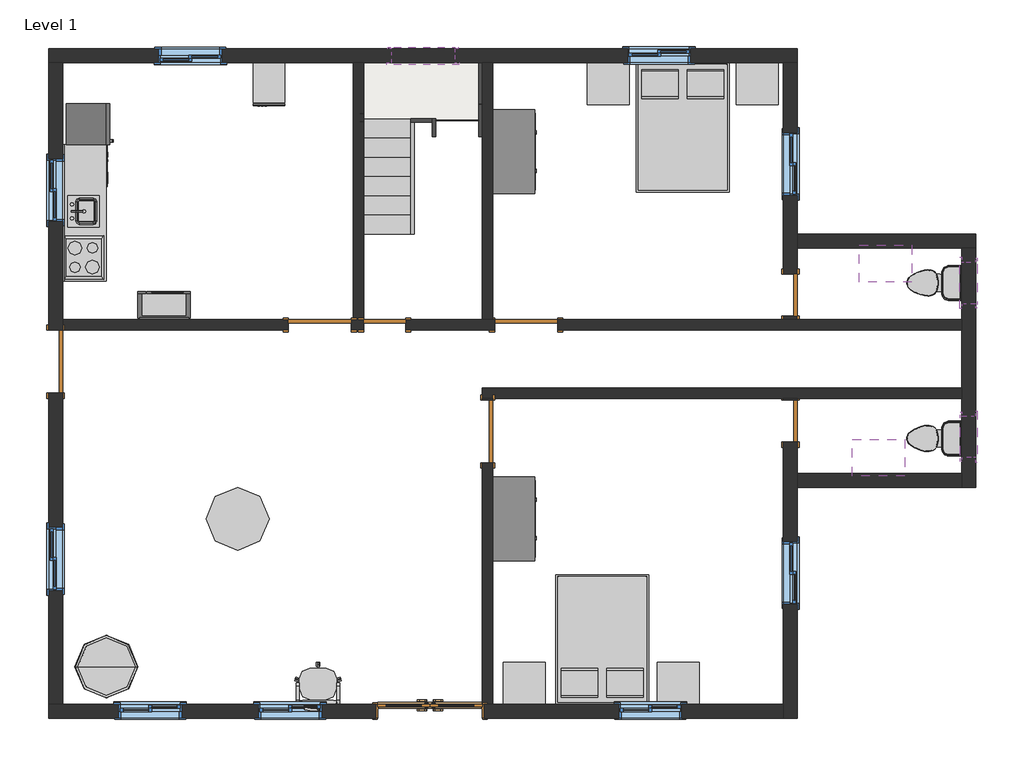
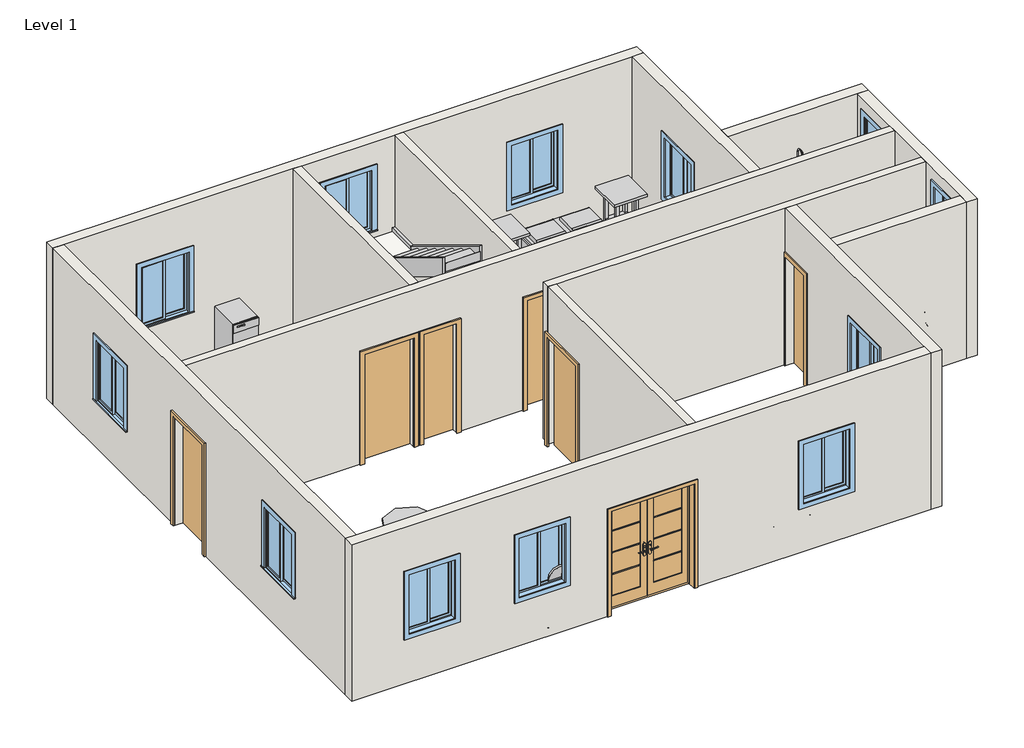
# One storey, incomplete: 13 walls, 12 furniture elements, 12 windows, 8 doors, 8 members, 6 proxies, 5 flow terminals, 2 stair flights, 1 slab.
# Revit data of these elements (continued)
# Element 23 (IfcFurniture, "Counter Top w Sink Hole : 24\" Depth") (continued)
#   Sink Opening Width = 1' - 4"
#   Phase Created = New Construction
#   Materials on its faces: "Counter Top"
# Elements 24, 25 (IfcFurniture, "Dresser : 48\" x 72\" x 24\"")
#   Phase Created = New Construction
#   Materials on its faces: "Laminate, Ivory, Matte", "Cherry", "Laminate - Ivory, Glossy"
# Element 26 (IfcFurniture, "Table-Dining Round w Chairs : 36\" Diameter")
#   Phase Created = New Construction
#   Materials on its faces: "Pine", "Laminate, Linen, Matte"
# Elements 27, 28, 29, 30 (IfcFurniture, "Table-Night Stand : 24\" x 24\" x 30\"")
#   Phase Created = New Construction
#   Materials on its faces: "Birch", "Laminate, Ivory, Matte"
# Element 31 (IfcFurniture, "Table-Round : 36\" Diameter")
#   Phase Created = New Construction
#   Materials on its faces: "Steel, Chrome Plated", "Birch"
# Elements 32, 33, 34, 35, 36, 37, 38, 39 (IfcMember, "Stringer - 2\" Width")
#   Phase Created = New Construction
# Element 40 (IfcSlab, "Non-Monolithic Landing")
#   Phase Created = New Construction
# Elements 41, 42 (IfcStairFlight, "2\" Tread 1\" Nosing 1/4\" Riser")
#   Phase Created = New Construction
# Elements 43, 44, 45, 46, 47, 48, 49, 50 (IfcWall, "Generic - 8\"")
#   Top Offset = 0' - 0"
#   Base Offset = 0' - 0"
#   Unconnected Height = 10' - 0"
#   wall height = 10' - 0"
#   Phase Created = New Construction
#   Base Constraint = Level 1
#   Materials on its faces: "Default Wall"
# Elements 51, 52, 53, 54, 55 (IfcWall, "inner wall")
#   Top Offset = 0' - 0"
#   Base Offset = 0' - 0"
#   Unconnected Height = 10' - 0"
#   wall height = 10' - 0"
#   Phase Created = New Construction
#   Base Constraint = Level 1
#   Materials on its faces: "Default Wall"
# Element 56 (IfcWindow, "Slider with Trim : 36\" x 48\"")
#   Mark = "1"
#   Phase Created = New Construction
#   Materials on its faces: "Sash", "Trim", "Glass"
# Element 57 (IfcWindow, "Slider with Trim : 36\" x 48\"")
#   Mark = "2"
#   Phase Created = New Construction
#   Materials on its faces: "Sash", "Trim", "Glass"
# Element 58 (IfcWindow, "Slider with Trim : 36\" x 48\"")
#   Mark = "3"
#   Phase Created = New Construction
#   Materials on its faces: "Sash", "Trim", "Glass"
# Element 59 (IfcWindow, "Slider with Trim : 36\" x 48\"")
#   Mark = "4"
#   Phase Created = New Construction
#   Materials on its faces: "Sash", "Trim", "Glass"
# Element 60 (IfcWindow, "Slider with Trim : 36\" x 48\"")
#   Mark = "5"
#   Phase Created = New Construction
#   Materials on its faces: "Sash", "Trim", "Glass"
# Element 61 (IfcWindow, "Slider with Trim : 36\" x 48\"")
#   Mark = "6"
#   Phase Created = New Construction
#   Materials on its faces: "Sash", "Trim", "Glass"
# Element 62 (IfcWindow, "Slider with Trim : 36\" x 48\"")
#   Mark = "7"
#   Phase Created = New Construction
#   Materials on its faces: "Sash", "Trim", "Glass"
# Element 63 (IfcWindow, "Slider with Trim : 36\" x 48\"")
#   Mark = "8"
#   Phase Created = New Construction
#   Materials on its faces: "Sash", "Trim", "Glass"
# Element 64 (IfcWindow, "Slider with Trim : 36\" x 48\"")
#   Mark = "9"
#   Phase Created = New Construction
#   Materials on its faces: "Sash", "Trim", "Glass"
# Element 65 (IfcWindow, "Slider with Trim : 36\" x 48\"")
#   Mark = "10"
#   Phase Created = New Construction
#   Materials on its faces: "Sash", "Trim", "Glass"
# Element 66 (IfcWindow, "Transom with Trim : 24\" x 24\"")
#   Mark = "11"
#   Phase Created = New Construction
#   Materials on its faces: "Sash", "Trim", "Glass"
# Element 67 (IfcWindow, "Transom with Trim : 24\" x 24\"")
#   Mark = "12"
#   Phase Created = New Construction
#   Materials on its faces: "Sash", "Trim", "Glass"
# Materials
#   "Plastic, Opaque Black": class "Plastic", colour RGB 0 0 0, transparency 0.7, Description = "Plastic, generic, opaque black", Cost = 0
#   "Steel, Paint Finish, Ivory, Matte": class "Metal", colour RGB 247 247 239, transparency 0, Description = "Steel, paint finish, ivory, matte", Cost = 0
#   "Steel, Chrome Plated": class "Metal", colour RGB 17 17 17, transparency 0, Description = "Chromiuim plated steel", Cost = 0
#   "Steel, Polished": class "Metal", colour RGB 57 57 57, transparency 0, Description = "Polished steel", Cost = 0
#   "Steel, Paint Finish, Ivory, Glossy": class "Metal", colour RGB 247 247 239, transparency 0, Description = "Steel, paint finish, ivory, glossy", Cost = 0
#   "Cabinets": colour RGB 249 249 249, transparency 0
#   "Cabinets - Handles": class "Metal", colour RGB 57 57 57, transparency 0
#   "Laminate, Ivory, Matte": class "Plastic", colour RGB 247 247 239, transparency 0, Description = "Plastic Laminate - Ivory, Matte", Cost = 0
#   "Cherry": class "Wood", colour RGB 226 177 128, transparency 0, Description = "Prunus Serotina", Cost = 0
#   "Glass": class "Glass", colour RGB 0 128 192, transparency 0.75, Description = "Soda Lime Glass", Cost = 0
#   "Aluminum": class "Metal", colour RGB 247 247 247, transparency 0, Description = "Aluminum 6061", Cost = 0
#   "Door - Panel": class "Wood", colour RGB 210 159 95, transparency 0
#   "Door - Frame": colour RGB 118 70 51, transparency 0
#   "Porcelain, Linen": class "Ceramic", colour RGB 249 239 230, transparency 0, Description = "Porcelain, linen", Cost = 0
#   "Laminate, Linen, Matte": class "Plastic", colour RGB 249 239 230, transparency 0, Description = "Plastic Laminate - Linen, Matte", Cost = 0
#   "Birch": class "Wood", colour RGB 224 178 126, transparency 0, Description = "Betula Alleghaniensis", Cost = 0
#   "Linen, White": class "Textile", colour RGB 247 247 239, transparency 0, Description = "Linen, white", Cost = 0
#   "Textile - Slate Blue": class "Fabric", colour RGB 98 102 118, transparency 0
#   "Laminate - Ivory, Glossy": colour RGB 247 247 239, transparency 0
#   "Pine": class "Wood", colour RGB 223 192 134, transparency 0, Description = "Pinus Echinata", Cost = 0
#   "Sash": class "Wood", colour RGB 224 178 126, transparency 0
#   "Trim": class "Wood", colour RGB 224 178 126, transparency 0
#   "Counter Top": class "Wood", colour RGB 226 177 128, transparency 0
#   "Default Wall": colour RGB 128 128 128, transparency 0
# Room at (-12590.439, 7905.42) mm, phase "New Construction", upper level "Level 1", upper offset 10' - 0", lower offset 0' - 0"
#   Number = "1"
#   Name = "KITCHEN AREA"
# Room at (-6185.849, 7905.42) mm, phase "New Construction", upper level "Level 1", upper offset 10' - 0", lower offset 0' - 0"
#   Number = "2"
#   Name = "BED ROOM"
# Room at (-11623.364, 3854.653) mm, phase "New Construction", upper level "Level 1", upper offset 10' - 0", lower offset 0' - 0"
#   Number = "3"
# Room at (-6185.849, 3289.005) mm, phase "New Construction", upper level "Level 1", upper offset 10' - 0", lower offset 0' - 0"
#   Number = "4"
#   Name = "BED ROOM"
# Room at (-2682.483, 4551.161) mm, phase "New Construction", upper level "Level 1", upper offset 10' - 0", lower offset 0' - 0"
#   Number = "5"
#   Name = "WC+BATH"
# Room at (-3010.924, 6643.264) mm, phase "New Construction", upper level "Level 1", upper offset 10' - 0", lower offset 0' - 0"
#   Number = "6"
#   Name = "WC+BATH"
